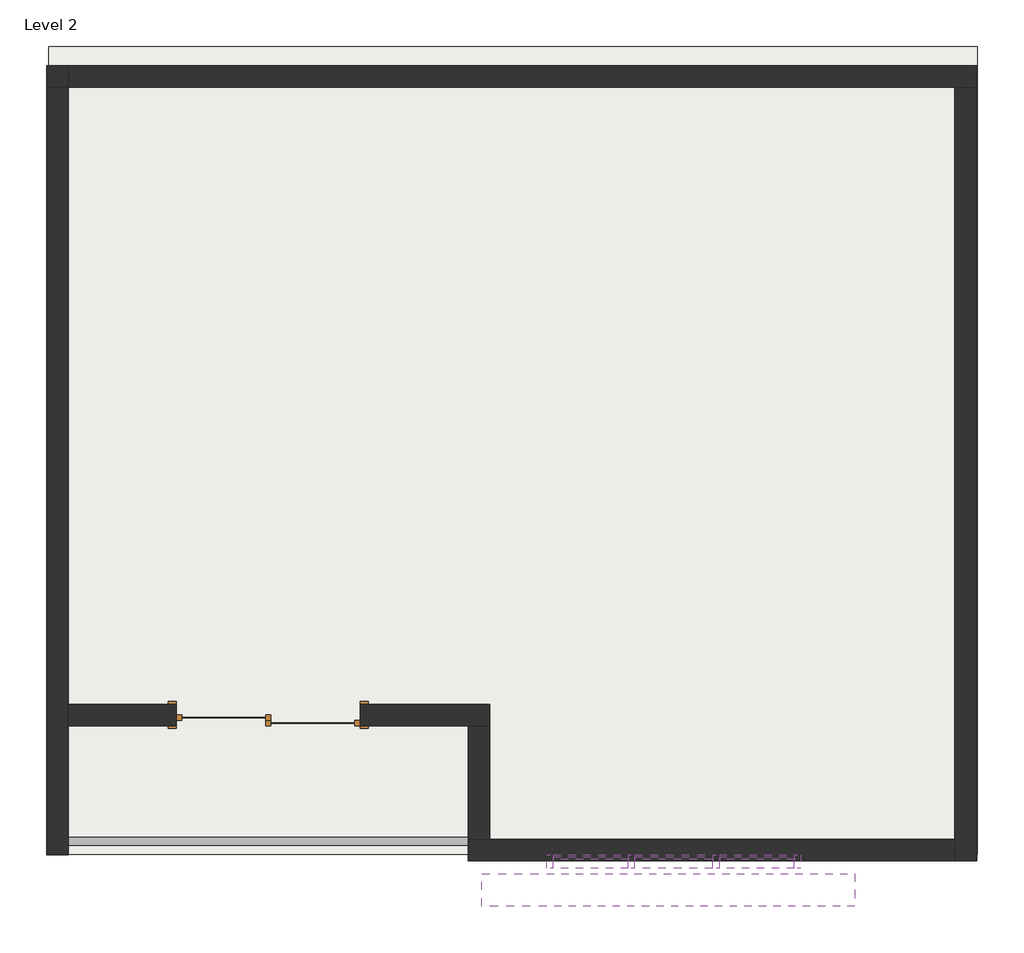
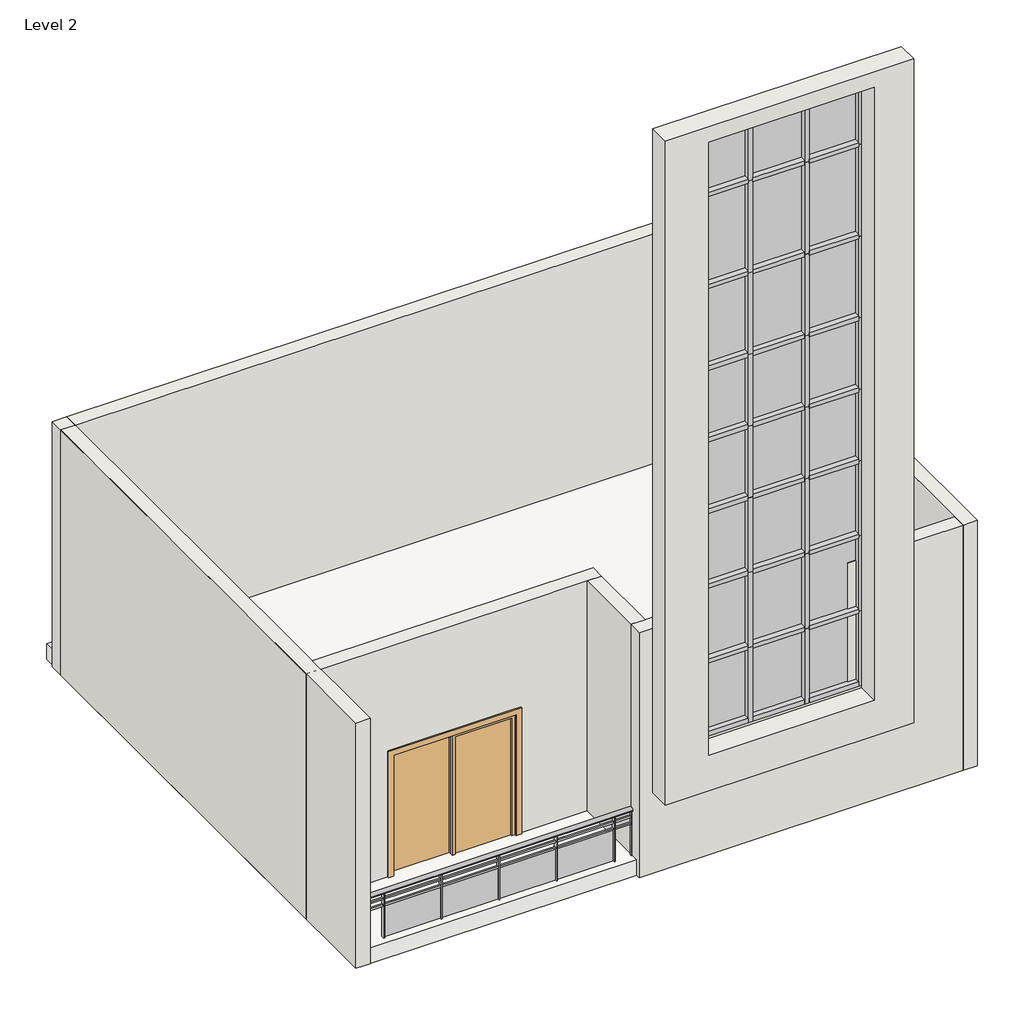
# One storey: 59 members, 24 plates, 8 walls, 1 door, 1 railing, 1 roof.
"""IFC4 building model written with IfcOpenShell, lengths in millimetres."""

from ifc_helpers import new_model, si_unit, point, frame, origin, place, context, project, spatial, polyline, ellipse_curve, trimmed, outline, extrude, faceted_brep, transform, mapped, element, save
from ifc_brep_helpers import plane_surface, extruded_surface, advanced_brep
from components import door_076b30e0, member_4a3a2774, member_824a4a8d, member_2b49869a, member_a715cb85, member_b546c93c, member_a689c7fc, member_3a8a164c, member_94a221ea, member_02c0e4c4, member_c4de40ee, member_75074519, member_c6627131, system_panel_glazed_05e8e754, system_panel_glazed_ccf5e832, system_panel_glazed_c5f71645, system_panel_glazed_22ff1419, system_panel_glazed_993ccbbe, system_panel_glazed_8af8589b, system_panel_glazed_62f7861e, system_panel_glazed_840f75dd, system_panel_glazed_68e8fd94, system_panel_glazed_fc79919b, system_panel_glazed_0dd3fac7, system_panel_glazed_09521bd2, walls_1_walls_1_c9c6bd33

model = new_model("IFC4")

# Units and contexts
model_context = context("Model", 3, world=origin())
ifc_project = project(units=[si_unit("LENGTHUNIT", "METRE", prefix="MILLI")], contexts=[model_context])

# Site, building, storey
site = spatial("IfcSite", under=ifc_project)
building = spatial("IfcBuilding", under=site)
storey = spatial("IfcBuildingStorey", under=building, Name="Level 2", Elevation=3657.6)

# Door
placement = place(None, origin())
door_shape = door_076b30e0(model_context)
element("IfcDoor", 1, ObjectType="Door-Double-Sliding : 68\" x 80\"", at=placement, inside=storey, context=model_context, shape_type="MappedRepresentation", body=[
    mapped(door_shape, transform((-12373.432922, 6303.7117654, 3657.6), x_axis=(-1.0, 0.0, 0.0), y_axis=(0.0, -1.0, 0.0), z_axis=(0.0, 0.0, 1.0))),
])

# Members
member_shape = member_4a3a2774(model_context)
element("IfcMember", 2, ObjectType="Rectangular Mullion : 2.5\" x 5\" rectangular", at=placement, inside=storey, context=model_context, shape_type="MappedRepresentation", body=[
    mapped(member_shape, transform((-8197.2495887, 4798.7617654, 13563.6), x_axis=(0.0, 0.0, 1.0), y_axis=(0.0, -1.0, 0.0), z_axis=(1.0, 0.0, 0.0))),
])
element("IfcMember", 3, ObjectType="Rectangular Mullion : 2.5\" x 5\" rectangular", at=placement, inside=storey, context=model_context, shape_type="MappedRepresentation", body=[
    mapped(member_shape, transform((-8197.2495887, 4798.7617654, 12192.0), x_axis=(0.0, 0.0, 1.0), y_axis=(0.0, -1.0, 0.0), z_axis=(1.0, 0.0, 0.0))),
])
element("IfcMember", 4, ObjectType="Rectangular Mullion : 2.5\" x 5\" rectangular", at=placement, inside=storey, context=model_context, shape_type="MappedRepresentation", body=[
    mapped(member_shape, transform((-8197.2495887, 4798.7617654, 10972.8), x_axis=(0.0, 0.0, 1.0), y_axis=(0.0, -1.0, 0.0), z_axis=(1.0, 0.0, 0.0))),
])
element("IfcMember", 5, ObjectType="Rectangular Mullion : 2.5\" x 5\" rectangular", at=placement, inside=storey, context=model_context, shape_type="MappedRepresentation", body=[
    mapped(member_shape, transform((-8197.2495887, 4798.7617654, 9906.0), x_axis=(0.0, 0.0, 1.0), y_axis=(0.0, -1.0, 0.0), z_axis=(1.0, 0.0, 0.0))),
])
element("IfcMember", 6, ObjectType="Rectangular Mullion : 2.5\" x 5\" rectangular", at=placement, inside=storey, context=model_context, shape_type="MappedRepresentation", body=[
    mapped(member_shape, transform((-8197.2495887, 4798.7617654, 8839.2), x_axis=(0.0, 0.0, 1.0), y_axis=(0.0, -1.0, 0.0), z_axis=(1.0, 0.0, 0.0))),
])
element("IfcMember", 7, ObjectType="Rectangular Mullion : 2.5\" x 5\" rectangular", at=placement, inside=storey, context=model_context, shape_type="MappedRepresentation", body=[
    mapped(member_shape, transform((-8197.2495887, 4798.7617654, 7721.6), x_axis=(0.0, 0.0, 1.0), y_axis=(0.0, -1.0, 0.0), z_axis=(1.0, 0.0, 0.0))),
])
element("IfcMember", 8, ObjectType="Rectangular Mullion : 2.5\" x 5\" rectangular", at=placement, inside=storey, context=model_context, shape_type="MappedRepresentation", body=[
    mapped(member_shape, transform((-8197.2495887, 4798.7617654, 6604.0), x_axis=(0.0, 0.0, 1.0), y_axis=(0.0, -1.0, 0.0), z_axis=(1.0, 0.0, 0.0))),
])
member_2_shape = member_824a4a8d(model_context)
element("IfcMember", 9, ObjectType="Rectangular Mullion : 2.5\" x 5\" rectangular", at=placement, inside=storey, context=model_context, shape_type="MappedRepresentation", body=[
    mapped(member_2_shape, transform((-8165.4995887, 4798.7617654, 12192.0), x_axis=(1.0, 0.0, 0.0), y_axis=(0.0, -1.0, 0.0), z_axis=(0.0, 0.0, -1.0))),
])
element("IfcMember", 10, ObjectType="Rectangular Mullion : 2.5\" x 5\" rectangular", at=placement, inside=storey, context=model_context, shape_type="MappedRepresentation", body=[
    mapped(member_2_shape, transform((-8961.3662553, 4798.7617654, 12192.0), x_axis=(1.0, 0.0, 0.0), y_axis=(0.0, -1.0, 0.0), z_axis=(0.0, 0.0, -1.0))),
])
member_3_shape = member_2b49869a(model_context)
element("IfcMember", 11, ObjectType="Rectangular Mullion : 2.5\" x 5\" rectangular", at=placement, inside=storey, context=model_context, shape_type="MappedRepresentation", body=[
    mapped(member_3_shape, transform((-8165.4995887, 4798.7617654, 10972.8), x_axis=(1.0, 0.0, 0.0), y_axis=(0.0, -1.0, 0.0), z_axis=(0.0, 0.0, -1.0))),
])
element("IfcMember", 12, ObjectType="Rectangular Mullion : 2.5\" x 5\" rectangular", at=placement, inside=storey, context=model_context, shape_type="MappedRepresentation", body=[
    mapped(member_3_shape, transform((-8961.3662553, 4798.7617654, 10972.8), x_axis=(1.0, 0.0, 0.0), y_axis=(0.0, -1.0, 0.0), z_axis=(0.0, 0.0, -1.0))),
])
member_4_shape = member_a715cb85(model_context)
element("IfcMember", 13, ObjectType="Rectangular Mullion : 2.5\" x 5\" rectangular", at=placement, inside=storey, context=model_context, shape_type="MappedRepresentation", body=[
    mapped(member_4_shape, transform((-8165.4995887, 4798.7617654, 8839.2), x_axis=(1.0, 0.0, 0.0), y_axis=(0.0, -1.0, 0.0), z_axis=(0.0, 0.0, -1.0))),
])
element("IfcMember", 14, ObjectType="Rectangular Mullion : 2.5\" x 5\" rectangular", at=placement, inside=storey, context=model_context, shape_type="MappedRepresentation", body=[
    mapped(member_4_shape, transform((-8165.4995887, 4798.7617654, 9906.0), x_axis=(1.0, 0.0, 0.0), y_axis=(0.0, -1.0, 0.0), z_axis=(0.0, 0.0, -1.0))),
])
element("IfcMember", 15, ObjectType="Rectangular Mullion : 2.5\" x 5\" rectangular", at=placement, inside=storey, context=model_context, shape_type="MappedRepresentation", body=[
    mapped(member_4_shape, transform((-8961.3662553, 4798.7617654, 8839.2), x_axis=(1.0, 0.0, 0.0), y_axis=(0.0, -1.0, 0.0), z_axis=(0.0, 0.0, -1.0))),
])
element("IfcMember", 16, ObjectType="Rectangular Mullion : 2.5\" x 5\" rectangular", at=placement, inside=storey, context=model_context, shape_type="MappedRepresentation", body=[
    mapped(member_4_shape, transform((-8961.3662553, 4798.7617654, 9906.0), x_axis=(1.0, 0.0, 0.0), y_axis=(0.0, -1.0, 0.0), z_axis=(0.0, 0.0, -1.0))),
])
member_5_shape = member_b546c93c(model_context)
element("IfcMember", 17, ObjectType="Rectangular Mullion : 2.5\" x 5\" rectangular", at=placement, inside=storey, context=model_context, shape_type="MappedRepresentation", body=[
    mapped(member_5_shape, transform((-8165.4995887, 4798.7617654, 6604.0), x_axis=(1.0, 0.0, 0.0), y_axis=(0.0, -1.0, 0.0), z_axis=(0.0, 0.0, -1.0))),
])
element("IfcMember", 18, ObjectType="Rectangular Mullion : 2.5\" x 5\" rectangular", at=placement, inside=storey, context=model_context, shape_type="MappedRepresentation", body=[
    mapped(member_5_shape, transform((-8165.4995887, 4798.7617654, 7721.6), x_axis=(1.0, 0.0, 0.0), y_axis=(0.0, -1.0, 0.0), z_axis=(0.0, 0.0, -1.0))),
])
element("IfcMember", 19, ObjectType="Rectangular Mullion : 2.5\" x 5\" rectangular", at=placement, inside=storey, context=model_context, shape_type="MappedRepresentation", body=[
    mapped(member_5_shape, transform((-8961.3662553, 4798.7617654, 6604.0), x_axis=(1.0, 0.0, 0.0), y_axis=(0.0, -1.0, 0.0), z_axis=(0.0, 0.0, -1.0))),
])
element("IfcMember", 20, ObjectType="Rectangular Mullion : 2.5\" x 5\" rectangular", at=placement, inside=storey, context=model_context, shape_type="MappedRepresentation", body=[
    mapped(member_5_shape, transform((-8961.3662553, 4798.7617654, 7721.6), x_axis=(1.0, 0.0, 0.0), y_axis=(0.0, -1.0, 0.0), z_axis=(0.0, 0.0, -1.0))),
])
element("IfcMember", 21, ObjectType="Rectangular Mullion : 2.5\" x 5\" rectangular", at=placement, inside=storey, context=model_context, shape_type="MappedRepresentation", body=[
    mapped(member_5_shape, transform((-8165.4995887, 4798.7617654, 5486.4), x_axis=(1.0, 0.0, 0.0), y_axis=(0.0, -1.0, 0.0), z_axis=(0.0, 0.0, -1.0))),
])
element("IfcMember", 22, ObjectType="Rectangular Mullion : 2.5\" x 5\" rectangular", at=placement, inside=storey, context=model_context, shape_type="MappedRepresentation", body=[
    mapped(member_5_shape, transform((-8961.3662553, 4798.7617654, 5486.4), x_axis=(1.0, 0.0, 0.0), y_axis=(0.0, -1.0, 0.0), z_axis=(0.0, 0.0, -1.0))),
])
member_6_shape = member_a689c7fc(model_context)
element("IfcMember", 23, ObjectType="Rectangular Mullion : 2.5\" x 5\" rectangular", at=placement, inside=storey, context=model_context, shape_type="MappedRepresentation", body=[
    mapped(member_6_shape, transform((-8929.6162553, 4798.7617654, 5486.4), x_axis=(0.0, 0.0, -1.0), y_axis=(0.0, -1.0, 0.0), z_axis=(-1.0, 0.0, 0.0))),
])
member_7_shape = member_3a8a164c(model_context)
element("IfcMember", 24, ObjectType="Rectangular Mullion : 2.5\" x 5\" rectangular", at=placement, inside=storey, context=model_context, shape_type="MappedRepresentation", body=[
    mapped(member_7_shape, transform((-7433.132922, 4798.7617654, 13563.6), x_axis=(0.0, 0.0, 1.0), y_axis=(0.0, -1.0, 0.0), z_axis=(1.0, 0.0, 0.0))),
])
element("IfcMember", 25, ObjectType="Rectangular Mullion : 2.5\" x 5\" rectangular", at=placement, inside=storey, context=model_context, shape_type="MappedRepresentation", body=[
    mapped(member_7_shape, transform((-8993.1162553, 4798.7617654, 13563.6), x_axis=(0.0, 0.0, 1.0), y_axis=(0.0, -1.0, 0.0), z_axis=(1.0, 0.0, 0.0))),
])
element("IfcMember", 26, ObjectType="Rectangular Mullion : 2.5\" x 5\" rectangular", at=placement, inside=storey, context=model_context, shape_type="MappedRepresentation", body=[
    mapped(member_7_shape, transform((-7433.132922, 4798.7617654, 12192.0), x_axis=(0.0, 0.0, 1.0), y_axis=(0.0, -1.0, 0.0), z_axis=(1.0, 0.0, 0.0))),
])
element("IfcMember", 27, ObjectType="Rectangular Mullion : 2.5\" x 5\" rectangular", at=placement, inside=storey, context=model_context, shape_type="MappedRepresentation", body=[
    mapped(member_7_shape, transform((-8993.1162553, 4798.7617654, 12192.0), x_axis=(0.0, 0.0, 1.0), y_axis=(0.0, -1.0, 0.0), z_axis=(1.0, 0.0, 0.0))),
])
element("IfcMember", 28, ObjectType="Rectangular Mullion : 2.5\" x 5\" rectangular", at=placement, inside=storey, context=model_context, shape_type="MappedRepresentation", body=[
    mapped(member_7_shape, transform((-7433.132922, 4798.7617654, 10972.8), x_axis=(0.0, 0.0, 1.0), y_axis=(0.0, -1.0, 0.0), z_axis=(1.0, 0.0, 0.0))),
])
element("IfcMember", 29, ObjectType="Rectangular Mullion : 2.5\" x 5\" rectangular", at=placement, inside=storey, context=model_context, shape_type="MappedRepresentation", body=[
    mapped(member_7_shape, transform((-8993.1162553, 4798.7617654, 10972.8), x_axis=(0.0, 0.0, 1.0), y_axis=(0.0, -1.0, 0.0), z_axis=(1.0, 0.0, 0.0))),
])
element("IfcMember", 30, ObjectType="Rectangular Mullion : 2.5\" x 5\" rectangular", at=placement, inside=storey, context=model_context, shape_type="MappedRepresentation", body=[
    mapped(member_7_shape, transform((-7433.132922, 4798.7617654, 9906.0), x_axis=(0.0, 0.0, 1.0), y_axis=(0.0, -1.0, 0.0), z_axis=(1.0, 0.0, 0.0))),
])
element("IfcMember", 31, ObjectType="Rectangular Mullion : 2.5\" x 5\" rectangular", at=placement, inside=storey, context=model_context, shape_type="MappedRepresentation", body=[
    mapped(member_7_shape, transform((-8993.1162553, 4798.7617654, 9906.0), x_axis=(0.0, 0.0, 1.0), y_axis=(0.0, -1.0, 0.0), z_axis=(1.0, 0.0, 0.0))),
])
element("IfcMember", 32, ObjectType="Rectangular Mullion : 2.5\" x 5\" rectangular", at=placement, inside=storey, context=model_context, shape_type="MappedRepresentation", body=[
    mapped(member_7_shape, transform((-7433.132922, 4798.7617654, 8839.2), x_axis=(0.0, 0.0, 1.0), y_axis=(0.0, -1.0, 0.0), z_axis=(1.0, 0.0, 0.0))),
])
element("IfcMember", 33, ObjectType="Rectangular Mullion : 2.5\" x 5\" rectangular", at=placement, inside=storey, context=model_context, shape_type="MappedRepresentation", body=[
    mapped(member_7_shape, transform((-8993.1162553, 4798.7617654, 8839.2), x_axis=(0.0, 0.0, 1.0), y_axis=(0.0, -1.0, 0.0), z_axis=(1.0, 0.0, 0.0))),
])
element("IfcMember", 34, ObjectType="Rectangular Mullion : 2.5\" x 5\" rectangular", at=placement, inside=storey, context=model_context, shape_type="MappedRepresentation", body=[
    mapped(member_7_shape, transform((-7433.132922, 4798.7617654, 7721.6), x_axis=(0.0, 0.0, 1.0), y_axis=(0.0, -1.0, 0.0), z_axis=(1.0, 0.0, 0.0))),
])
element("IfcMember", 35, ObjectType="Rectangular Mullion : 2.5\" x 5\" rectangular", at=placement, inside=storey, context=model_context, shape_type="MappedRepresentation", body=[
    mapped(member_7_shape, transform((-8993.1162553, 4798.7617654, 7721.6), x_axis=(0.0, 0.0, 1.0), y_axis=(0.0, -1.0, 0.0), z_axis=(1.0, 0.0, 0.0))),
])
element("IfcMember", 36, ObjectType="Rectangular Mullion : 2.5\" x 5\" rectangular", at=placement, inside=storey, context=model_context, shape_type="MappedRepresentation", body=[
    mapped(member_7_shape, transform((-7433.132922, 4798.7617654, 6604.0), x_axis=(0.0, 0.0, 1.0), y_axis=(0.0, -1.0, 0.0), z_axis=(1.0, 0.0, 0.0))),
])
element("IfcMember", 37, ObjectType="Rectangular Mullion : 2.5\" x 5\" rectangular", at=placement, inside=storey, context=model_context, shape_type="MappedRepresentation", body=[
    mapped(member_7_shape, transform((-8993.1162553, 4798.7617654, 6604.0), x_axis=(0.0, 0.0, 1.0), y_axis=(0.0, -1.0, 0.0), z_axis=(1.0, 0.0, 0.0))),
])
member_8_shape = member_94a221ea(model_context)
element("IfcMember", 38, ObjectType="Rectangular Mullion : 2.5\" x 5\" rectangular", at=placement, inside=storey, context=model_context, shape_type="MappedRepresentation", body=[
    mapped(member_8_shape, transform((-8133.7495887, 4798.7617654, 5486.4), x_axis=(0.0, 0.0, -1.0), y_axis=(0.0, -1.0, 0.0), z_axis=(-1.0, 0.0, 0.0))),
])
element("IfcMember", 39, ObjectType="Rectangular Mullion : 2.5\" x 5\" rectangular", at=placement, inside=storey, context=model_context, shape_type="MappedRepresentation", body=[
    mapped(member_8_shape, transform((-9693.732922, 4798.7617654, 5486.4), x_axis=(0.0, 0.0, -1.0), y_axis=(0.0, -1.0, 0.0), z_axis=(-1.0, 0.0, 0.0))),
])
member_9_shape = member_02c0e4c4(model_context)
element("IfcMember", 40, ObjectType="Rectangular Mullion : 2.5\" x 5\" rectangular", at=placement, inside=storey, context=model_context, shape_type="MappedRepresentation", body=[
    mapped(member_9_shape, transform((-7369.632922, 4798.7617654, 6604.0), x_axis=(1.0, 0.0, 0.0), y_axis=(0.0, -1.0, 0.0), z_axis=(0.0, 0.0, -1.0))),
])
element("IfcMember", 41, ObjectType="Rectangular Mullion : 2.5\" x 5\" rectangular", at=placement, inside=storey, context=model_context, shape_type="MappedRepresentation", body=[
    mapped(member_9_shape, transform((-7369.632922, 4798.7617654, 7721.6), x_axis=(1.0, 0.0, 0.0), y_axis=(0.0, -1.0, 0.0), z_axis=(0.0, 0.0, -1.0))),
])
member_10_shape = member_c4de40ee(model_context)
element("IfcMember", 42, ObjectType="Rectangular Mullion : 2.5\" x 5\" rectangular", at=placement, inside=storey, context=model_context, shape_type="MappedRepresentation", body=[
    mapped(member_10_shape, transform((-7369.632922, 4798.7617654, 8839.2), x_axis=(1.0, 0.0, 0.0), y_axis=(0.0, -1.0, 0.0), z_axis=(0.0, 0.0, -1.0))),
])
element("IfcMember", 43, ObjectType="Rectangular Mullion : 2.5\" x 5\" rectangular", at=placement, inside=storey, context=model_context, shape_type="MappedRepresentation", body=[
    mapped(member_10_shape, transform((-7369.632922, 4798.7617654, 9906.0), x_axis=(1.0, 0.0, 0.0), y_axis=(0.0, -1.0, 0.0), z_axis=(0.0, 0.0, -1.0))),
])
member_11_shape = member_75074519(model_context)
element("IfcMember", 44, ObjectType="Rectangular Mullion : 2.5\" x 5\" rectangular", at=placement, inside=storey, context=model_context, shape_type="MappedRepresentation", body=[
    mapped(member_11_shape, transform((-7369.632922, 4798.7617654, 10972.8), x_axis=(1.0, 0.0, 0.0), y_axis=(0.0, -1.0, 0.0), z_axis=(0.0, 0.0, -1.0))),
])
member_12_shape = member_c6627131(model_context)
element("IfcMember", 45, ObjectType="Rectangular Mullion : 2.5\" x 5\" rectangular", at=placement, inside=storey, context=model_context, shape_type="MappedRepresentation", body=[
    mapped(member_12_shape, transform((-7369.632922, 4798.7617654, 12192.0), x_axis=(1.0, 0.0, 0.0), y_axis=(0.0, -1.0, 0.0), z_axis=(0.0, 0.0, -1.0))),
])
element("IfcMember", 46, ObjectType="Rectangular Mullion : 2.5\" x 5\" rectangular", at=placement, inside=storey, context=model_context, shape_type="MappedRepresentation", body=[
    mapped(member_9_shape, transform((-7369.632922, 4798.7617654, 5486.4), x_axis=(1.0, 0.0, 0.0), y_axis=(0.0, -1.0, 0.0), z_axis=(0.0, 0.0, -1.0))),
])
element("IfcMember", 47, ObjectType="Rectangular Mullion : 2.5\" x 5\" rectangular", at=placement, inside=storey, context=model_context, shape_type="MappedRepresentation", body=[
    mapped(member_9_shape, transform((-9757.232922, 4798.7617654, 6604.0), x_axis=(-1.0, 0.0, 0.0), y_axis=(0.0, -1.0, 0.0), z_axis=(0.0, 0.0, 1.0))),
])
element("IfcMember", 48, ObjectType="Rectangular Mullion : 2.5\" x 5\" rectangular", at=placement, inside=storey, context=model_context, shape_type="MappedRepresentation", body=[
    mapped(member_9_shape, transform((-9757.232922, 4798.7617654, 7721.6), x_axis=(-1.0, 0.0, 0.0), y_axis=(0.0, -1.0, 0.0), z_axis=(0.0, 0.0, 1.0))),
])
element("IfcMember", 49, ObjectType="Rectangular Mullion : 2.5\" x 5\" rectangular", at=placement, inside=storey, context=model_context, shape_type="MappedRepresentation", body=[
    mapped(member_9_shape, transform((-9757.232922, 4798.7617654, 8839.2), x_axis=(-1.0, 0.0, 0.0), y_axis=(0.0, -1.0, 0.0), z_axis=(0.0, 0.0, 1.0))),
])
element("IfcMember", 50, ObjectType="Rectangular Mullion : 2.5\" x 5\" rectangular", at=placement, inside=storey, context=model_context, shape_type="MappedRepresentation", body=[
    mapped(member_10_shape, transform((-9757.232922, 4798.7617654, 9906.0), x_axis=(-1.0, 0.0, 0.0), y_axis=(0.0, -1.0, 0.0), z_axis=(0.0, 0.0, 1.0))),
])
element("IfcMember", 51, ObjectType="Rectangular Mullion : 2.5\" x 5\" rectangular", at=placement, inside=storey, context=model_context, shape_type="MappedRepresentation", body=[
    mapped(member_10_shape, transform((-9757.232922, 4798.7617654, 10972.8), x_axis=(-1.0, 0.0, 0.0), y_axis=(0.0, -1.0, 0.0), z_axis=(0.0, 0.0, 1.0))),
])
element("IfcMember", 52, ObjectType="Rectangular Mullion : 2.5\" x 5\" rectangular", at=placement, inside=storey, context=model_context, shape_type="MappedRepresentation", body=[
    mapped(member_11_shape, transform((-9757.232922, 4798.7617654, 12192.0), x_axis=(-1.0, 0.0, 0.0), y_axis=(0.0, -1.0, 0.0), z_axis=(0.0, 0.0, 1.0))),
])
element("IfcMember", 53, ObjectType="Rectangular Mullion : 2.5\" x 5\" rectangular", at=placement, inside=storey, context=model_context, shape_type="MappedRepresentation", body=[
    mapped(member_12_shape, transform((-9757.232922, 4798.7617654, 13563.6), x_axis=(-1.0, 0.0, 0.0), y_axis=(0.0, -1.0, 0.0), z_axis=(0.0, 0.0, 1.0))),
])
element("IfcMember", 54, ObjectType="Rectangular Mullion : 2.5\" x 5\" rectangular", at=placement, inside=storey, context=model_context, shape_type="MappedRepresentation", body=[
    mapped(member_4_shape, transform((-8165.4995887, 4798.7617654, 13563.6), x_axis=(1.0, 0.0, 0.0), y_axis=(0.0, -1.0, 0.0), z_axis=(0.0, 0.0, -1.0))),
])
element("IfcMember", 55, ObjectType="Rectangular Mullion : 2.5\" x 5\" rectangular", at=placement, inside=storey, context=model_context, shape_type="MappedRepresentation", body=[
    mapped(member_4_shape, transform((-8961.3662553, 4798.7617654, 13563.6), x_axis=(1.0, 0.0, 0.0), y_axis=(0.0, -1.0, 0.0), z_axis=(0.0, 0.0, -1.0))),
])
element("IfcMember", 56, ObjectType="Rectangular Mullion : 2.5\" x 5\" rectangular", at=placement, inside=storey, context=model_context, shape_type="MappedRepresentation", body=[
    mapped(member_8_shape, transform((-8993.1162553, 4798.7617654, 14630.4), x_axis=(0.0, 0.0, 1.0), y_axis=(0.0, -1.0, 0.0), z_axis=(1.0, 0.0, 0.0))),
])
element("IfcMember", 57, ObjectType="Rectangular Mullion : 2.5\" x 5\" rectangular", at=placement, inside=storey, context=model_context, shape_type="MappedRepresentation", body=[
    mapped(member_8_shape, transform((-7433.132922, 4798.7617654, 14630.4), x_axis=(0.0, 0.0, 1.0), y_axis=(0.0, -1.0, 0.0), z_axis=(1.0, 0.0, 0.0))),
])
element("IfcMember", 58, ObjectType="Rectangular Mullion : 2.5\" x 5\" rectangular", at=placement, inside=storey, context=model_context, shape_type="MappedRepresentation", body=[
    mapped(member_6_shape, transform((-8197.2495887, 4798.7617654, 14630.4), x_axis=(0.0, 0.0, 1.0), y_axis=(0.0, -1.0, 0.0), z_axis=(1.0, 0.0, 0.0))),
])
element("IfcMember", 59, ObjectType="Rectangular Mullion : 2.5\" x 5\" rectangular", at=placement, inside=storey, context=model_context, shape_type="MappedRepresentation", body=[
    mapped(member_10_shape, transform((-7369.632922, 4798.7617654, 13563.6), x_axis=(1.0, 0.0, 0.0), y_axis=(0.0, -1.0, 0.0), z_axis=(0.0, 0.0, -1.0))),
])
element("IfcMember", 60, ObjectType="Rectangular Mullion : 2.5\" x 5\" rectangular", at=placement, inside=storey, context=model_context, shape_type="MappedRepresentation", body=[
    mapped(member_10_shape, transform((-9757.232922, 4798.7617654, 14630.4), x_axis=(-1.0, 0.0, 0.0), y_axis=(0.0, -1.0, 0.0), z_axis=(0.0, 0.0, 1.0))),
])

# Plates
system_panel_glazed_shape = system_panel_glazed_05e8e754(model_context)
element("IfcPlate", 61, ObjectType="System Panel : Glazed", at=placement, inside=storey, context=model_context, shape_type="MappedRepresentation", body=[
    mapped(system_panel_glazed_shape, transform((-8563.432922, 4798.7617654, 12223.75), x_axis=(1.0, 0.0, 0.0), y_axis=(0.0, 1.0, 0.0), z_axis=(0.0, 0.0, 1.0))),
])
system_panel_glazed_2_shape = system_panel_glazed_ccf5e832(model_context)
element("IfcPlate", 62, ObjectType="System Panel : Glazed", at=placement, inside=storey, context=model_context, shape_type="MappedRepresentation", body=[
    mapped(system_panel_glazed_2_shape, transform((-8563.432922, 4798.7617654, 11004.55), x_axis=(1.0, 0.0, 0.0), y_axis=(0.0, 1.0, 0.0), z_axis=(0.0, 0.0, 1.0))),
])
system_panel_glazed_3_shape = system_panel_glazed_c5f71645(model_context)
element("IfcPlate", 63, ObjectType="System Panel : Glazed", at=placement, inside=storey, context=model_context, shape_type="MappedRepresentation", body=[
    mapped(system_panel_glazed_3_shape, transform((-8563.432922, 4798.7617654, 9937.75), x_axis=(1.0, 0.0, 0.0), y_axis=(0.0, 1.0, 0.0), z_axis=(0.0, 0.0, 1.0))),
])
element("IfcPlate", 64, ObjectType="System Panel : Glazed", at=placement, inside=storey, context=model_context, shape_type="MappedRepresentation", body=[
    mapped(system_panel_glazed_3_shape, transform((-8563.432922, 4798.7617654, 8870.95), x_axis=(1.0, 0.0, 0.0), y_axis=(0.0, 1.0, 0.0), z_axis=(0.0, 0.0, 1.0))),
])
system_panel_glazed_4_shape = system_panel_glazed_22ff1419(model_context)
element("IfcPlate", 65, ObjectType="System Panel : Glazed", at=placement, inside=storey, context=model_context, shape_type="MappedRepresentation", body=[
    mapped(system_panel_glazed_4_shape, transform((-8563.432922, 4798.7617654, 7753.35), x_axis=(1.0, 0.0, 0.0), y_axis=(0.0, 1.0, 0.0), z_axis=(0.0, 0.0, 1.0))),
])
element("IfcPlate", 66, ObjectType="System Panel : Glazed", at=placement, inside=storey, context=model_context, shape_type="MappedRepresentation", body=[
    mapped(system_panel_glazed_4_shape, transform((-8563.432922, 4798.7617654, 6635.75), x_axis=(1.0, 0.0, 0.0), y_axis=(0.0, 1.0, 0.0), z_axis=(0.0, 0.0, 1.0))),
])
system_panel_glazed_5_shape = system_panel_glazed_993ccbbe(model_context)
element("IfcPlate", 67, ObjectType="System Panel : Glazed", at=placement, inside=storey, context=model_context, shape_type="MappedRepresentation", body=[
    mapped(system_panel_glazed_5_shape, transform((-8563.432922, 4798.7617654, 5549.9), x_axis=(1.0, 0.0, 0.0), y_axis=(0.0, 1.0, 0.0), z_axis=(0.0, 0.0, 1.0))),
])
system_panel_glazed_6_shape = system_panel_glazed_8af8589b(model_context)
element("IfcPlate", 68, ObjectType="System Panel : Glazed", at=placement, inside=storey, context=model_context, shape_type="MappedRepresentation", body=[
    mapped(system_panel_glazed_6_shape, transform((-9343.4245887, 4798.7617654, 5549.9), x_axis=(1.0, 0.0, 0.0), y_axis=(0.0, 1.0, 0.0), z_axis=(0.0, 0.0, 1.0))),
])
element("IfcPlate", 69, ObjectType="System Panel : Glazed", at=placement, inside=storey, context=model_context, shape_type="MappedRepresentation", body=[
    mapped(system_panel_glazed_6_shape, transform((-7783.4412553, 4798.7617654, 5549.9), x_axis=(1.0, 0.0, 0.0), y_axis=(0.0, 1.0, 0.0), z_axis=(0.0, 0.0, 1.0))),
])
system_panel_glazed_7_shape = system_panel_glazed_62f7861e(model_context)
element("IfcPlate", 70, ObjectType="System Panel : Glazed", at=placement, inside=storey, context=model_context, shape_type="MappedRepresentation", body=[
    mapped(system_panel_glazed_7_shape, transform((-9343.4245887, 4798.7617654, 12223.75), x_axis=(1.0, 0.0, 0.0), y_axis=(0.0, 1.0, 0.0), z_axis=(0.0, 0.0, 1.0))),
])
element("IfcPlate", 71, ObjectType="System Panel : Glazed", at=placement, inside=storey, context=model_context, shape_type="MappedRepresentation", body=[
    mapped(system_panel_glazed_7_shape, transform((-7783.4412553, 4798.7617654, 12223.75), x_axis=(1.0, 0.0, 0.0), y_axis=(0.0, 1.0, 0.0), z_axis=(0.0, 0.0, 1.0))),
])
system_panel_glazed_8_shape = system_panel_glazed_840f75dd(model_context)
element("IfcPlate", 72, ObjectType="System Panel : Glazed", at=placement, inside=storey, context=model_context, shape_type="MappedRepresentation", body=[
    mapped(system_panel_glazed_8_shape, transform((-9343.4245887, 4798.7617654, 11004.55), x_axis=(1.0, 0.0, 0.0), y_axis=(0.0, 1.0, 0.0), z_axis=(0.0, 0.0, 1.0))),
])
element("IfcPlate", 73, ObjectType="System Panel : Glazed", at=placement, inside=storey, context=model_context, shape_type="MappedRepresentation", body=[
    mapped(system_panel_glazed_8_shape, transform((-7783.4412553, 4798.7617654, 11004.55), x_axis=(1.0, 0.0, 0.0), y_axis=(0.0, 1.0, 0.0), z_axis=(0.0, 0.0, 1.0))),
])
system_panel_glazed_9_shape = system_panel_glazed_68e8fd94(model_context)
element("IfcPlate", 74, ObjectType="System Panel : Glazed", at=placement, inside=storey, context=model_context, shape_type="MappedRepresentation", body=[
    mapped(system_panel_glazed_9_shape, transform((-9343.4245887, 4798.7617654, 9937.75), x_axis=(1.0, 0.0, 0.0), y_axis=(0.0, 1.0, 0.0), z_axis=(0.0, 0.0, 1.0))),
])
element("IfcPlate", 75, ObjectType="System Panel : Glazed", at=placement, inside=storey, context=model_context, shape_type="MappedRepresentation", body=[
    mapped(system_panel_glazed_9_shape, transform((-7783.4412553, 4798.7617654, 9937.75), x_axis=(1.0, 0.0, 0.0), y_axis=(0.0, 1.0, 0.0), z_axis=(0.0, 0.0, 1.0))),
])
element("IfcPlate", 76, ObjectType="System Panel : Glazed", at=placement, inside=storey, context=model_context, shape_type="MappedRepresentation", body=[
    mapped(system_panel_glazed_9_shape, transform((-9343.4245887, 4798.7617654, 8870.95), x_axis=(1.0, 0.0, 0.0), y_axis=(0.0, 1.0, 0.0), z_axis=(0.0, 0.0, 1.0))),
])
element("IfcPlate", 77, ObjectType="System Panel : Glazed", at=placement, inside=storey, context=model_context, shape_type="MappedRepresentation", body=[
    mapped(system_panel_glazed_9_shape, transform((-7783.4412553, 4798.7617654, 8870.95), x_axis=(1.0, 0.0, 0.0), y_axis=(0.0, 1.0, 0.0), z_axis=(0.0, 0.0, 1.0))),
])
system_panel_glazed_10_shape = system_panel_glazed_fc79919b(model_context)
element("IfcPlate", 78, ObjectType="System Panel : Glazed", at=placement, inside=storey, context=model_context, shape_type="MappedRepresentation", body=[
    mapped(system_panel_glazed_10_shape, transform((-9343.4245887, 4798.7617654, 7753.35), x_axis=(1.0, 0.0, 0.0), y_axis=(0.0, 1.0, 0.0), z_axis=(0.0, 0.0, 1.0))),
])
element("IfcPlate", 79, ObjectType="System Panel : Glazed", at=placement, inside=storey, context=model_context, shape_type="MappedRepresentation", body=[
    mapped(system_panel_glazed_10_shape, transform((-7783.4412553, 4798.7617654, 7753.35), x_axis=(1.0, 0.0, 0.0), y_axis=(0.0, 1.0, 0.0), z_axis=(0.0, 0.0, 1.0))),
])
element("IfcPlate", 80, ObjectType="System Panel : Glazed", at=placement, inside=storey, context=model_context, shape_type="MappedRepresentation", body=[
    mapped(system_panel_glazed_10_shape, transform((-9343.4245887, 4798.7617654, 6635.75), x_axis=(1.0, 0.0, 0.0), y_axis=(0.0, 1.0, 0.0), z_axis=(0.0, 0.0, 1.0))),
])
element("IfcPlate", 81, ObjectType="System Panel : Glazed", at=placement, inside=storey, context=model_context, shape_type="MappedRepresentation", body=[
    mapped(system_panel_glazed_10_shape, transform((-7783.4412553, 4798.7617654, 6635.75), x_axis=(1.0, 0.0, 0.0), y_axis=(0.0, 1.0, 0.0), z_axis=(0.0, 0.0, 1.0))),
])
system_panel_glazed_11_shape = system_panel_glazed_0dd3fac7(model_context)
element("IfcPlate", 82, ObjectType="System Panel : Glazed", at=placement, inside=storey, context=model_context, shape_type="MappedRepresentation", body=[
    mapped(system_panel_glazed_11_shape, transform((-9343.4245887, 4798.7617654, 13595.35), x_axis=(1.0, 0.0, 0.0), y_axis=(0.0, 1.0, 0.0), z_axis=(0.0, 0.0, 1.0))),
])
element("IfcPlate", 83, ObjectType="System Panel : Glazed", at=placement, inside=storey, context=model_context, shape_type="MappedRepresentation", body=[
    mapped(system_panel_glazed_11_shape, transform((-7783.4412553, 4798.7617654, 13595.35), x_axis=(1.0, 0.0, 0.0), y_axis=(0.0, 1.0, 0.0), z_axis=(0.0, 0.0, 1.0))),
])
system_panel_glazed_12_shape = system_panel_glazed_09521bd2(model_context)
element("IfcPlate", 84, ObjectType="System Panel : Glazed", at=placement, inside=storey, context=model_context, shape_type="MappedRepresentation", body=[
    mapped(system_panel_glazed_12_shape, transform((-8563.432922, 4798.7617654, 13595.35), x_axis=(1.0, 0.0, 0.0), y_axis=(0.0, 1.0, 0.0), z_axis=(0.0, 0.0, 1.0))),
])

# Railing
element("IfcRailing", 85, ObjectType="Glass Panel - Bottom Fill", at=placement, inside=storey, context=model_context, shape_type="SolidModel", body=[
    advanced_brep(
    [(-14253.032922, 5027.3617654, 4572.0), (-14253.032922, 4951.1617654, 4572.0), (-10493.832922, 5027.3617654, 4572.0), (-10493.832922, 4951.1617654, 4572.0)],
    [
        (0, 1, ellipse_curve(frame((-14253.032922, 4989.2617654, 4572.0), z_axis=(-1.0, 0.0, 0.0), x_axis=(0.0, -1.0, 0.0)), 38.1, 28.575)),
        (1, 0, ellipse_curve(frame((-14253.032922, 4989.2617654, 4572.0), z_axis=(-1.0, 0.0, 0.0), x_axis=(0.0, -1.0, 0.0)), 38.1, 28.575)),
        (2, 3, ellipse_curve(frame((-10493.832922, 4989.2617654, 4572.0), z_axis=(1.0, 0.0, 0.0), x_axis=(0.0, -1.0, 0.0)), 38.1, 28.575)),
        (3, 2, ellipse_curve(frame((-10493.832922, 4989.2617654, 4572.0), z_axis=(1.0, 0.0, 0.0), x_axis=(0.0, -1.0, 0.0)), 38.1, 28.575)),
        (0, 2),
        (3, 1),
    ],
    [
        plane_surface(frame((-14253.032922, 4989.2617654, 4572.0), z_axis=(-1.0, 0.0, 0.0), x_axis=(0.0, 1.0, 0.0))),
        plane_surface(frame((-10493.832922, 4989.2617654, 4572.0), z_axis=(1.0, 0.0, 0.0), x_axis=(0.0, 1.0, 0.0))),
        extruded_surface(trimmed(ellipse_curve(frame((-10493.832922, 4989.2617654, 4572.0), z_axis=(-1.0, 0.0, 0.0), x_axis=(0.0, -1.0, 0.0)), 38.1, 28.575), [point((-10493.832922, 5027.3617654, 4572.0))], [point((-10493.832922, 4951.1617654, 4572.0))], True, "CARTESIAN"), (-3759.2000000000007, 0.0, 0.0), 3759.2000000000007),
        extruded_surface(trimmed(ellipse_curve(frame((-10493.832922, 4989.2617654, 4572.0), z_axis=(-1.0, 0.0, 0.0), x_axis=(0.0, -1.0, 0.0)), 38.1, 28.575), [point((-10493.832922, 4951.1617654, 4572.0))], [point((-10493.832922, 5027.3617654, 4572.0))], True, "CARTESIAN"), (-3759.2000000000007, 0.0, 0.0), 3759.2000000000007),
    ],
    [
        (0, [[1, 2]]),
        (1, [[3, 4]]),
        (2, [[-1, 5, -4, 6]]),
        (3, [[-2, -6, -3, -5]]),
    ],
),
    extrude(outline(polyline([(-14253.032922, 4976.5617654), (-14253.032922, 5001.9617654), (-10493.832922, 5001.9617654), (-10493.832922, 4976.5617654), (-14253.032922, 4976.5617654)])), frame((0.0, 0.0, 4457.7), z_axis=(0.0, 0.0, 1.0), x_axis=(1.0, 0.0, 0.0)), (0.0, 0.0, 1.0), 25.4),
    extrude(outline(polyline([(-14253.032922, 4976.5617654), (-14253.032922, 5001.9617654), (-10493.832922, 5001.9617654), (-10493.832922, 4976.5617654), (-14253.032922, 4976.5617654)])), frame((0.0, 0.0, 4356.1), z_axis=(0.0, 0.0, 1.0), x_axis=(1.0, 0.0, 0.0)), (0.0, 0.0, 1.0), 25.4),
    extrude(outline(polyline([(-10754.182922, 4963.8617654), (-10754.182922, 5014.6617654), (-10741.482922, 5014.6617654), (-10741.482922, 4963.8617654), (-10754.182922, 4963.8617654)])), frame((0.0, 0.0, 3657.6), z_axis=(0.0, 0.0, 1.0), x_axis=(1.0, 0.0, 0.0)), (0.0, 0.0, 1.0), 885.6788223),
    extrude(outline(polyline([(-11560.632922, 4995.7969224), (-10747.832922, 4995.7969224), (-10747.832922, 4989.4469224), (-11560.632922, 4989.4469224), (-11560.632922, 4995.7969224)])), frame((0.0, 0.0, 3759.2), z_axis=(0.0, 0.0, 1.0), x_axis=(1.0, 0.0, 0.0)), (0.0, 0.0, 1.0), 596.9),
    extrude(outline(polyline([(-11566.982922, 4963.8617654), (-11566.982922, 5014.6617654), (-11554.282922, 5014.6617654), (-11554.282922, 4963.8617654), (-11566.982922, 4963.8617654)])), frame((0.0, 0.0, 3657.6), z_axis=(0.0, 0.0, 1.0), x_axis=(1.0, 0.0, 0.0)), (0.0, 0.0, 1.0), 885.6788223),
    extrude(outline(polyline([(-12373.432922, 4995.7969224), (-11560.632922, 4995.7969224), (-11560.632922, 4989.4469224), (-12373.432922, 4989.4469224), (-12373.432922, 4995.7969224)])), frame((0.0, 0.0, 3759.2), z_axis=(0.0, 0.0, 1.0), x_axis=(1.0, 0.0, 0.0)), (0.0, 0.0, 1.0), 596.9),
    extrude(outline(polyline([(-12379.782922, 4963.8617654), (-12379.782922, 5014.6617654), (-12367.082922, 5014.6617654), (-12367.082922, 4963.8617654), (-12379.782922, 4963.8617654)])), frame((0.0, 0.0, 3657.6), z_axis=(0.0, 0.0, 1.0), x_axis=(1.0, 0.0, 0.0)), (0.0, 0.0, 1.0), 885.6788223),
    extrude(outline(polyline([(-13186.232922, 4995.7969224), (-12373.432922, 4995.7969224), (-12373.432922, 4989.4469224), (-13186.232922, 4989.4469224), (-13186.232922, 4995.7969224)])), frame((0.0, 0.0, 3759.2), z_axis=(0.0, 0.0, 1.0), x_axis=(1.0, 0.0, 0.0)), (0.0, 0.0, 1.0), 596.9),
    extrude(outline(polyline([(-13192.582922, 4963.8617654), (-13192.582922, 5014.6617654), (-13179.882922, 5014.6617654), (-13179.882922, 4963.8617654), (-13192.582922, 4963.8617654)])), frame((0.0, 0.0, 3657.6), z_axis=(0.0, 0.0, 1.0), x_axis=(1.0, 0.0, 0.0)), (0.0, 0.0, 1.0), 885.6788223),
    extrude(outline(polyline([(-13999.032922, 4995.7969224), (-13186.232922, 4995.7969224), (-13186.232922, 4989.4469224), (-13999.032922, 4989.4469224), (-13999.032922, 4995.7969224)])), frame((0.0, 0.0, 3759.2), z_axis=(0.0, 0.0, 1.0), x_axis=(1.0, 0.0, 0.0)), (0.0, 0.0, 1.0), 596.9),
    extrude(outline(polyline([(-14005.382922, 4963.8617654), (-14005.382922, 5014.6617654), (-13992.682922, 5014.6617654), (-13992.682922, 4963.8617654), (-14005.382922, 4963.8617654)])), frame((0.0, 0.0, 3657.6), z_axis=(0.0, 0.0, 1.0), x_axis=(1.0, 0.0, 0.0)), (0.0, 0.0, 1.0), 885.6788223),
    extrude(outline(polyline([(-10506.532922, 4979.7367654), (-10506.532922, 4998.7867654), (-10487.482922, 4998.7867654), (-10487.482922, 4979.7367654), (-10506.532922, 4979.7367654)])), frame((0.0, 0.0, 3657.6), z_axis=(0.0, 0.0, 1.0), x_axis=(1.0, 0.0, 0.0)), (0.0, 0.0, 1.0), 885.6788223),
    extrude(outline(polyline([(-14259.382922, 4979.7367654), (-14259.382922, 4998.7867654), (-14240.332922, 4998.7867654), (-14240.332922, 4979.7367654), (-14259.382922, 4979.7367654)])), frame((0.0, 0.0, 3657.6), z_axis=(0.0, 0.0, 1.0), x_axis=(1.0, 0.0, 0.0)), (0.0, 0.0, 1.0), 885.6788223),
])

# Roof
element("IfcRoof", 86, ObjectType="Generic - 9\"", at=placement, inside=storey, context=model_context, shape_type="SweptSolid", body=[
    extrude(outline(polyline([(-14435.2593035, 12460.3935836), (-5710.3593035, 12460.3935836), (-5710.3593035, 4865.7935836), (-10301.4093035, 4865.7935836), (-14435.2593035, 4865.7935836), (-14435.2593035, 12460.3935836)])), frame((0.0, 0.0, 3657.6), z_axis=(0.0, 0.0, 1.0), x_axis=(1.0, 0.0, 0.0)), (0.0, 0.0, 1.0), 228.6),
])

# Walls
element("IfcWall", 87, ObjectType="Generic - 8\"", at=placement, inside=storey, context=model_context, shape_type="Brep", body=[
    faceted_brep([(-14253.032922, 6075.1117654, 3657.6), (-14253.032922, 6278.3117654, 3657.6), (-14253.032922, 12075.8617654, 3657.6), (-14253.032922, 12279.0617654, 3657.6), (-14253.032922, 12279.0617654, 7315.2), (-14253.032922, 12075.8617654, 7315.2), (-14253.032922, 6278.3117654, 7315.2), (-14253.032922, 6075.1117654, 7315.2), (-14456.232922, 6075.1117654, 3657.6), (-14456.232922, 6075.1117654, 7315.2), (-14456.232922, 12279.0617654, 7315.2), (-14456.232922, 12279.0617654, 3657.6), (-14456.232922, 12075.8617654, 3657.6)], [[[0, 1, 2, 3, 4, 5, 6, 7]], [[8, 9, 10, 11, 12]], [[3, 2, 1, 0, 8, 12, 11]], [[7, 6, 5, 4, 10, 9]], [[4, 3, 11, 10]], [[0, 7, 9, 8]]]),
])
element("IfcWall", 88, ObjectType="Generic - 8\"", at=placement, inside=storey, context=model_context, shape_type="Brep", body=[
    faceted_brep([(-14253.032922, 12075.8617654, 3657.6), (-5921.832922, 12075.8617654, 3657.6), (-5718.632922, 12075.8617654, 3657.6), (-5718.632922, 12075.8617654, 7315.2), (-5921.832922, 12075.8617654, 7315.2), (-14253.032922, 12075.8617654, 7315.2), (-14253.032922, 12279.0617654, 3657.6), (-14253.032922, 12279.0617654, 7315.2), (-5718.632922, 12279.0617654, 7315.2), (-5718.632922, 12279.0617654, 3657.6), (-5921.832922, 12279.0617654, 3657.6)], [[[0, 1, 2, 3, 4, 5]], [[6, 7, 8, 9, 10]], [[2, 1, 0, 6, 10, 9]], [[5, 4, 3, 8, 7]], [[3, 2, 9, 8]], [[0, 5, 7, 6]]]),
])
element("IfcWall", 89, ObjectType="Generic - 8\"", at=placement, inside=storey, context=model_context, shape_type="Brep", body=[
    faceted_brep([(-5921.832922, 12075.8617654, 3657.6), (-5921.832922, 5008.3117654, 3657.6), (-5921.832922, 4805.1117654, 3657.6), (-5921.832922, 4805.1117654, 7315.2), (-5921.832922, 5008.3117654, 7315.2), (-5921.832922, 12075.8617654, 7315.2), (-5718.632922, 12075.8617654, 3657.6), (-5718.632922, 12075.8617654, 7315.2), (-5718.632922, 4805.1117654, 7315.2), (-5718.632922, 4805.1117654, 3657.6)], [[[0, 1, 2, 3, 4, 5]], [[6, 7, 8, 9]], [[2, 1, 0, 6, 9]], [[5, 4, 3, 8, 7]], [[0, 5, 7, 6]], [[3, 2, 9, 8]]]),
])
element("IfcWall", 90, ObjectType="Generic - 8\"", at=placement, inside=storey, context=model_context, shape_type="Brep", body=[
    faceted_brep([(-5921.832922, 5008.3117654, 3657.6), (-10290.632922, 5008.3117654, 3657.6), (-10493.832922, 5008.3117654, 3657.6), (-10493.832922, 5008.3117654, 7315.2), (-10290.632922, 5008.3117654, 7315.2), (-9884.232922, 5008.3117654, 7315.2), (-9884.232922, 5008.3117654, 5486.4), (-7547.432922, 5008.3117654, 5486.4), (-7547.432922, 5008.3117654, 7315.2), (-5921.832922, 5008.3117654, 7315.2), (-5921.832922, 4805.1117654, 3657.6), (-5921.832922, 4805.1117654, 7315.2), (-7547.432922, 4805.1117654, 7315.2), (-7547.432922, 4805.1117654, 5486.4), (-9884.232922, 4805.1117654, 5486.4), (-9884.232922, 4805.1117654, 7315.2), (-10493.832922, 4805.1117654, 7315.2), (-10493.832922, 4805.1117654, 3657.6)], [[[0, 1, 2, 3, 4, 5, 6, 7, 8, 9]], [[10, 11, 12, 13, 14, 15, 16, 17]], [[0, 9, 11, 10]], [[3, 2, 17, 16]], [[2, 1, 0, 10, 17]], [[5, 4, 3, 16, 15]], [[6, 5, 15, 14]], [[7, 6, 14, 13]], [[8, 7, 13, 12]], [[9, 8, 12, 11]]]),
])
element("IfcWall", 91, ObjectType="Generic - 8\"", at=placement, inside=storey, context=model_context, shape_type="Brep", body=[
    faceted_brep([(-14253.032922, 6075.1117654, 3657.6), (-13237.032922, 6075.1117654, 3657.6), (-13237.032922, 6075.1117654, 5689.6), (-11509.832922, 6075.1117654, 5689.6), (-11509.832922, 6075.1117654, 3657.6), (-10493.832922, 6075.1117654, 3657.6), (-10290.632922, 6075.1117654, 3657.6), (-10290.632922, 6075.1117654, 7315.2), (-10493.832922, 6075.1117654, 7315.2), (-11459.032922, 6075.1117654, 7315.2), (-13186.232922, 6075.1117654, 7315.2), (-14253.032922, 6075.1117654, 7315.2), (-13237.032922, 6278.3117654, 5689.6), (-13237.032922, 6278.3117654, 3657.6), (-14253.032922, 6278.3117654, 3657.6), (-14253.032922, 6278.3117654, 7315.2), (-13186.232922, 6278.3117654, 7315.2), (-11459.032922, 6278.3117654, 7315.2), (-10290.632922, 6278.3117654, 7315.2), (-10290.632922, 6278.3117654, 3657.6), (-11509.832922, 6278.3117654, 3657.6), (-11509.832922, 6278.3117654, 5689.6)], [[[0, 1, 2, 3, 4, 5, 6, 7, 8, 9, 10, 11]], [[12, 13, 14, 15, 16, 17, 18, 19, 20, 21]], [[20, 19, 6, 5, 4]], [[14, 13, 1, 0]], [[11, 10, 9, 8, 7, 18, 17, 16, 15]], [[7, 6, 19, 18]], [[0, 11, 15, 14]], [[4, 3, 21, 20]], [[2, 1, 13, 12]], [[3, 2, 12, 21]]]),
])
element("IfcWall", 92, ObjectType="Generic - 8\"", at=placement, inside=storey, context=model_context, shape_type="SweptSolid", body=[
    extrude(outline(polyline([(-10493.832922, 5008.3117654), (-10493.832922, 6075.1117654), (-10290.632922, 6075.1117654), (-10290.632922, 5008.3117654), (-10493.832922, 5008.3117654)])), frame((0.0, 0.0, 3657.6), z_axis=(0.0, 0.0, 1.0), x_axis=(1.0, 0.0, 0.0)), (0.0, 0.0, 1.0), 3657.6),
])
element("IfcWall", 93, ObjectType="Generic - 8\"", at=placement, inside=storey, context=model_context, shape_type="SweptSolid", body=[
    extrude(outline(polyline([(-14253.032922, 12075.8617654), (-14253.032922, 4862.2617654), (-14456.232922, 4862.2617654), (-14456.232922, 12075.8617654), (-14253.032922, 12075.8617654)])), frame((0.0, 0.0, 3657.6), z_axis=(0.0, 0.0, 1.0), x_axis=(1.0, 0.0, 0.0)), (0.0, 0.0, 1.0), 3657.6),
])
walls_1_walls_1_shape = walls_1_walls_1_c9c6bd33(model_context)
element("IfcWall", 94, ObjectType="Walls 1 : Walls 1", at=placement, inside=storey, context=model_context, shape_type="MappedRepresentation", body=[
    mapped(walls_1_walls_1_shape, transform((0.0, 0.0, 0.0), x_axis=(1.0, 0.0, 0.0), y_axis=(0.0, 1.0, 0.0), z_axis=(0.0, 0.0, 1.0))),
])

save(model, "model.ifc")

# Revit data of these elements
# Type "Door-Double-Sliding : 68\" x 80\""
#   Type Mark = "8"
#   Construction Type Id = "opn-d45"
#   Assembly Code = "C1020"
#   Analytic Construction = "Wood frame, double glass door "
#   Thickness = 0' - 2"
#   Thermal Resistance (R) = 1.8150 (h·ft²·°F)/BTU
#   Heat Transfer Coefficient (U) = 0.5510 BTU/(h·ft²·°F)
#   Height = 6' - 8"
#   Rail Width = 0' - 2"
#   Stiles = 0' - 2"
#   Trim Projection Ext = 0' - 1"
#   Trim Projection Int = 0' - 1"
#   Trim Width = 0' - 3"
#   Width = 5' - 8"
#   Define Thermal Properties by = 1
#   Glazing = Glass
#   Panel Material = Wood - Birch - Solid Stained Light Low Gloss
#   Trim Material = Paint - Sienna
#   Visual Light Transmittance = 0
#   Solar Heat Gain Coefficient = 0
#   Function = (empty or 0)
#   Wall Closure = (empty or 0)
# Type "Rectangular Mullion : 2.5\" x 5\" rectangular"
#   built-in parameter 1007304 = 0.416667 (stored number, unit not read)
#   built-in parameter 1007301 = 0.104167 (stored number, unit not read)
#   built-in parameter 1007300 = 0.104167 (stored number, unit not read)
# Type "System Panel : Glazed"
#   Construction Type Id = "GSP4R"
#   Analytic Construction = "1/8 in Pilkington single glazing"
#   Visual Light Transmittance = 0.9
#   Solar Heat Gain Coefficient = 0.86
#   Heat Transfer Coefficient (U) = 1.18115 BTU/(h·ft²·°F)
# Type "Glass Panel - Bottom Fill"
#   Assembly Code = "C2010400"
#   built-in parameter 1008612 = 0.0416667 (stored number, unit not read)
#   built-in parameter 1008611 = 0.0416667 (stored number, unit not read)
#   built-in parameter 1008609 = 0.333333 (stored number, unit not read)
#   built-in parameter 1008604 = 0.166667 (stored number, unit not read)
#   built-in parameter 1008603 = 0.166667 (stored number, unit not read)
#   Railing Height = 3' - 0"
#   built-in parameter 1008630 = 2
#   built-in parameter 1008610 = 2
#   built-in parameter 1008618 = Baluster - Square : 3/4"
# Type "Generic - 9\""
#   Assembly Code = "B1020"
#   Layers, outside or top first: 0' - 9" no material (function 1)
# Type "Generic - 8\""
#   Assembly Code = "B2010"
#   Layers, outside or top first: 0' - 8" no material (function 1)
# Element 1 (IfcDoor, "Door-Double-Sliding : 68\" x 80\"")
#   Phase Created = New Construction
#   Materials on its faces: "Paint - Sienna", "Wood - Birch - Solid Stained Light Low Gloss", "Glass"
# Elements 2, 3, 4, 5, 6, 7, 8, 9, 10, 11, 12, 13, 14, 15, 16, 17, 18, 19, 20, 21, 22, 23, 24, 25, 26, 27, 28, 29, 30, 31, 32, 33, 34, 35, 36, 37, 38, 39, 40, 41, 42, 43, 44, 45, 46, 47, 48, 49, 50, 51, 52, 53, 54, 55, 56, 57, 58, 59, 60 (IfcMember, "Rectangular Mullion : 2.5\" x 5\" rectangular")
#   Phase Created = New Construction
#   Materials on its faces: "Aluminum"
# Elements 61, 62, 63, 64, 65, 66, 67, 68, 69, 70, 71, 72, 73, 74, 75, 76, 77, 78, 79, 80, 81, 82, 83, 84 (IfcPlate, "System Panel : Glazed")
#   Phase Created = New Construction
#   Materials on its faces: "Glass"
# Element 85 (IfcRailing, "Glass Panel - Bottom Fill")
#   Phase Created = New Construction
#   Materials on its faces: "Glass"
# Element 86 (IfcRoof, "Generic - 9\"")
#   built-in parameter 1001705 = 12.75 (stored number, unit not read)
#   built-in parameter 1001710 = 33615
#   Phase Created = New Construction
#   Materials on its faces: "Default Roof"
# Elements 87, 88, 89, 90, 91, 92, 93 (IfcWall, "Generic - 8\"")
#   Top Offset = 0' - 0"
#   Base Offset = 0' - 0"
#   Unconnected Height = 12' - 0"
#   wall height = 12' - 0"
#   Phase Created = New Construction
#   Base Constraint = Level 2
#   Materials on its faces: "Default Wall"
# Element 94 (IfcWall, "Walls 1 : Walls 1")
#   Phase Created = New Construction
#   Materials on its faces: "Default Wall"
# Materials
#   "Glass": class "Glass", colour RGB 0 128 192, transparency 0.75, Description = "Soda Lime Glass", Cost = 0
#   "Wood - Birch - Solid Stained Light Low Gloss": class "Wood", colour RGB 210 159 95, transparency 0, Cost = 0
#   "Paint - Sienna": colour RGB 118 70 51, transparency 0, Cost = 0
#   "Aluminum": class "Metal", colour RGB 247 247 247, transparency 0, Description = "Aluminum 6061", Cost = 0
#   "Default Roof": colour RGB 88 101 114, transparency 0
#   "Default Wall": colour RGB 128 128 128, transparency 0
